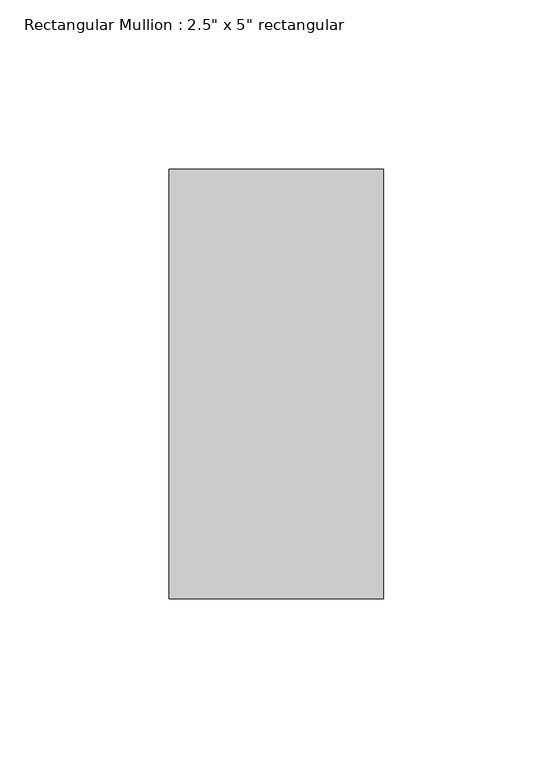
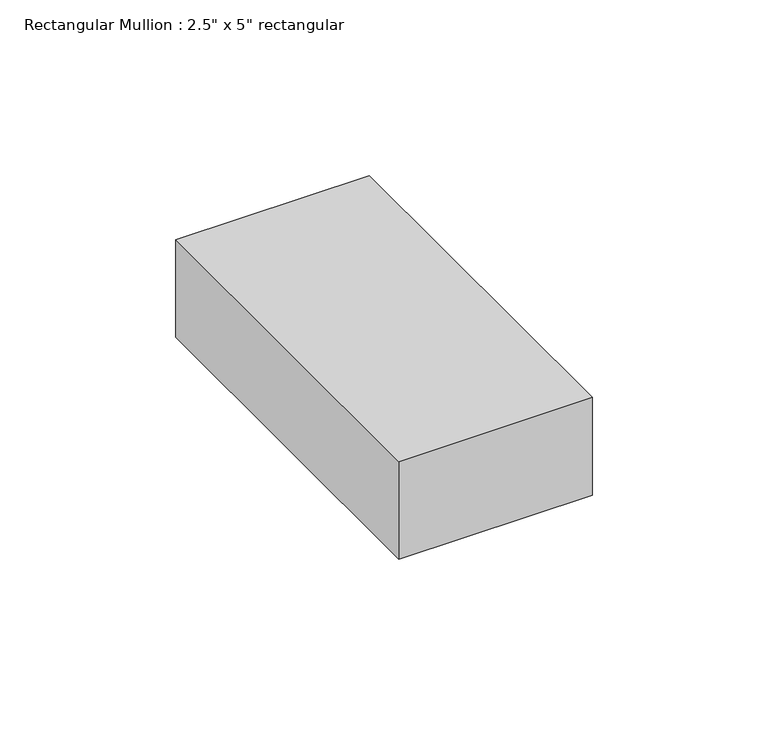
"""IFC4 building model written with IfcOpenShell, lengths in millimetres: member geometry."""

from ifc_helpers import new_model, si_unit, frame, origin, place, context, project, spatial, polyline, outline, extrude, source, transform, mapped, element, save


def member_d3f030c1(model_context):
    return source(origin(), model_context, "Body", "SweptSolid", [
        extrude(outline(polyline([(31.75, 63.5), (31.75, -63.5), (-31.75, -63.5), (-31.75, 63.5), (31.75, 63.5)])), frame((0.0, 0.0, -33.8666667), z_axis=(0.0, 0.0, 1.0), x_axis=(1.0, 0.0, 0.0)), (0.0, 0.0, 1.0), 33.8666667),
    ])


if __name__ == "__main__":
    model = new_model("IFC4")
    model_context = context("Model", 3, world=origin())
    ifc_project = project(units=[si_unit("LENGTHUNIT", "METRE", prefix="MILLI")], contexts=[model_context])
    site = spatial("IfcSite", under=ifc_project)
    building = spatial("IfcBuilding", under=site)
    placement = place(None, origin())
    member_shape = member_d3f030c1(model_context)
    element("IfcMember", 1, ObjectType="Rectangular Mullion : 2.5\" x 5\" rectangular", at=placement, inside=building, context=model_context, shape_type="MappedRepresentation", body=[
        mapped(member_shape, transform((0.0, 0.0, 0.0), x_axis=(1.0, 0.0, 0.0), y_axis=(0.0, 1.0, 0.0), z_axis=(0.0, 0.0, 1.0))),
    ])
    save(model, "model.ifc")

# Revit data of these elements
# Type "Rectangular Mullion : 2.5\" x 5\" rectangular"
#   built-in parameter 1007304 = 0.416667 (stored number, unit not read)
#   built-in parameter 1007301 = 0.104167 (stored number, unit not read)
#   built-in parameter 1007300 = 0.104167 (stored number, unit not read)
# Element 1 (IfcMember, "Rectangular Mullion : 2.5\" x 5\" rectangular")
#   Materials on its faces: "Aluminum"
# Materials
#   "Aluminum": class "Metal", colour RGB 247 247 247, transparency 0, Description = "Aluminum 6061", Cost = 0
